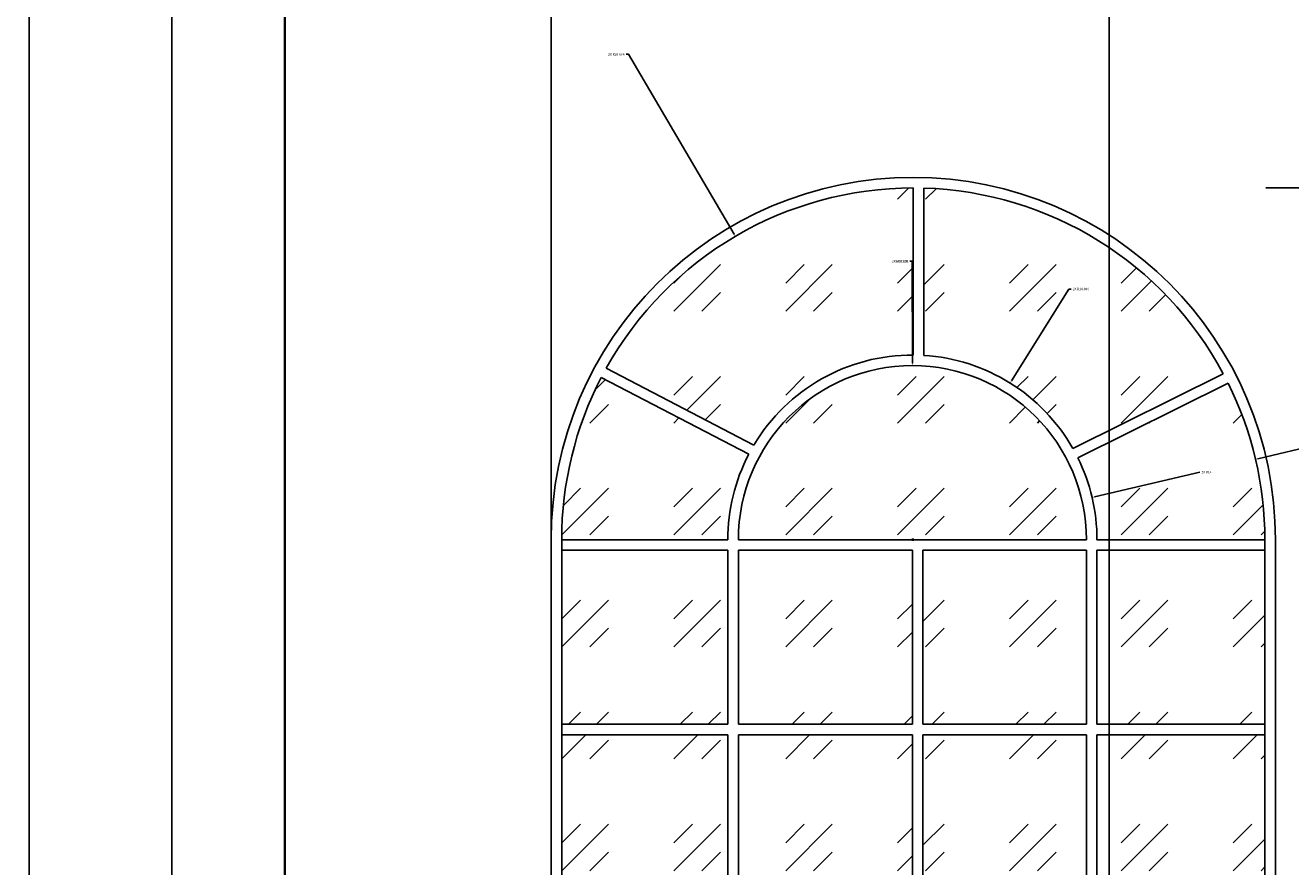
# Model space of a CAD drawing. Units: inches. Extents: x 93 to 565, y 123 to 656.
# Tile 15 of 18: x 418 to 513, y 518 to 582. Entities that reach past the tile are written whole.
import ezdxf

# ---------------------------------------------------------------- set-up
doc = ezdxf.new("R2010")
doc.units = ezdxf.units.IN
doc.header["$MEASUREMENT"] = 0
for name, color, linetype, lineweight in [('A-ANNO-DIMS', 2, 'Continuous', 18), ('A-ELEV', 7, 'Continuous', 35), ('A-GLAZ', 4, 'Continuous', 25)]:
    doc.layers.add(name, color=color, linetype=linetype, lineweight=lineweight)
doc.styles.get("Standard").update_dxf_attribs({"font": 'arial.ttf'})
doc.dimstyles.get("Standard").update_dxf_attribs({"dimtxt": 0.18, "dimasz": 0.18, "dimexe": 0.18, "dimexo": 0.0625, "dimgap": 0.09, "dimtad": 0, "dimtih": 1, "dimtoh": 1, "dimdec": 4, "dimzin": 0, "dimdsep": 46, "dimtxsty": 'Standard', "dimcen": 0.09, "dimadec": 0, "dimazin": 0, "dimtfac": 1, "dimtdec": 4, "dimtofl": 0, "dimtmove": 0, "dimatfit": 3, "dimfxl": 1, "dimtolj": 1, "dimtzin": 0, "dimarcsym": 0})

# ---------------------------------------------------------------- blocks, each defined once
blk = doc.blocks.new('WIN-ARCHED')
for p, q in [((26.666, 83.051), (26.666, 70.384)), ((27.466, 83.039), (27.466, 70.358)), ((3.385, 69.387), (14.576, 63.554)), ((3.006, 68.683), (14.186, 62.855)), ((50.181, 68.96), (38.77, 63.306)), ((50.548, 68.249), (39.145, 62.599)), ((0, 56.384), (12.6, 56.384)), ((0, 56.384), (0.2, 56.384)), ((0, 56.384), (0, 32.384)), ((13.4, 56.384), (39.8, 56.384)), ((40.6, 56.384), (53.333, 56.384)), ((0, 55.584), (12.6, 55.584)), ((12.6, 55.584), (12.6, 42.384)), ((13.4, 55.584), (13.4, 42.384)), ((13.4, 55.584), (26.6, 55.584)), ((26.6, 55.584), (26.6, 42.384)), ((27.4, 55.584), (27.4, 42.384)), ((27.4, 55.584), (39.8, 55.584)), ((39.8, 55.584), (39.8, 42.384)), ((40.6, 55.584), (40.6, 42.384)), ((40.6, 55.584), (53.333, 55.584)), ((0, 42.384), (12.6, 42.384)), ((13.4, 42.384), (26.6, 42.384)), ((27.4, 42.384), (39.8, 42.384)), ((40.6, 42.384), (53.333, 42.384)), ((0, 41.584), (12.6, 41.584)), ((12.6, 41.584), (12.6, 28.384)), ((13.4, 41.584), (13.4, 28.384)), ((13.4, 41.584), (26.6, 41.584)), ((26.6, 41.584), (26.6, 28.384)), ((27.4, 41.584), (27.4, 28.384)), ((27.4, 41.584), (39.8, 41.584)), ((39.8, 41.584), (39.8, 28.384)), ((40.6, 41.584), (40.6, 28.384)), ((40.6, 41.584), (53.333, 41.584)), ((0, 28.384), (12.6, 28.384)), ((13.4, 28.384), (26.6, 28.384)), ((27.4, 28.384), (39.8, 28.384)), ((40.6, 28.384), (53.333, 28.384)), ((0, 27.584), (12.6, 27.584)), ((12.6, 27.584), (12.6, 14.384)), ((13.4, 27.584), (13.4, 14.384)), ((13.4, 27.584), (26.6, 27.584)), ((26.6, 27.584), (26.6, 14.384)), ((27.4, 27.584), (27.4, 14.384)), ((27.4, 27.584), (39.8, 27.584)), ((39.8, 27.584), (39.8, 14.384)), ((40.6, 27.584), (40.6, 14.384)), ((40.6, 27.584), (53.333, 27.584)), ((0, 14.384), (12.6, 14.384)), ((0, 13.584), (12.6, 13.584)), ((12.6, 13.584), (12.6, 0)), ((13.4, 14.384), (26.6, 14.384)), ((13.4, 13.584), (13.4, 0)), ((13.4, 13.584), (26.6, 13.584)), ((26.6, 13.584), (26.6, 0)), ((27.4, 14.384), (39.8, 14.384)), ((27.4, 13.584), (27.4, 0)), ((27.4, 13.584), (39.8, 13.584)), ((39.8, 13.584), (39.8, 0)), ((40.6, 14.384), (53.333, 14.384)), ((40.6, 13.584), (40.6, 0)), ((40.6, 13.584), (53.333, 13.584))]:
    blk.add_line(p, q)
blk.add_lwpolyline([(53.333, 56.384), (53.333, 0), (0, 0), (0, 56.384)])
for centre, radius, start, end in [((26.666, 56.384), 26.666, 90, 150.81666), ((26.666, 56.384), 26.666, 28.13721, 88.28084), ((26.6, 56.384), 14, 89.72913, 149.19423), ((26.6, 56.384), 14, 29.63071, 86.45282), ((26.6, 56.384), 13.2, 0, 180), ((26.666, 56.384), 26.666, 152.53579, 180), ((26.666, 56.384), 26.666, 0, 26.41802), ((26.6, 56.384), 14, 152.47006, 180), ((26.6, 56.384), 14, 0, 26.35489)]:
    blk.add_arc(centre, radius, start, end)
blk = doc.blocks.new('*D20')
at = {"layer": 'A-ANNO-DIMS', "color": 0, "lineweight": -2, "transparency": 16777216}
for p, q in [((511.588, 569.373), (524.163, 569.373)), ((523.983, 569.193), (523.983, 528.031)), ((523.983, 486.502), (523.983, 527.664)), ((511.588, 486.322), (524.163, 486.322))]:
    blk.add_line(p, q, dxfattribs=at)
at = {"layer": 'A-ANNO-DIMS', "color": 0, "transparency": 16777216}
for points in [[(523.953, 569.193), (524.013, 569.193), (523.983, 569.373)], [(523.953, 486.502), (524.013, 486.502), (523.983, 486.322)]]:
    blk.add_solid(points, dxfattribs=at)
at = {"layer": 'Defpoints', "color": 0, "transparency": 16777216}
for p in [(511.526, 569.373), (523.983, 569.373), (511.526, 486.322)]:
    blk.add_point(p, dxfattribs=at)
at = {"layer": 'A-ANNO-DIMS', "color": 0, "transparency": 16777216, "insert": (523.983, 527.847), "char_height": 0.18, "attachment_point": 5}
blk.add_mtext('\\A1;ARCHED WINDOW 83 TYP.', dxfattribs=at)
blk = doc.blocks.new('*D26')
at = {"layer": 'A-ANNO-DIMS', "color": 0, "lineweight": -2, "transparency": 16777216}
for p, q in [((119.079, 519.162), (119.079, 656.135)), ((119.259, 655.955), (328.787, 655.955)), ((538.899, 655.955), (329.372, 655.955)), ((539.079, 630.467), (539.079, 656.135))]:
    blk.add_line(p, q, dxfattribs=at)
at = {"layer": 'A-ANNO-DIMS', "color": 0, "transparency": 16777216}
for points in [[(119.259, 655.985), (119.259, 655.925), (119.079, 655.955)], [(538.899, 655.985), (538.899, 655.925), (539.079, 655.955)]]:
    blk.add_solid(points, dxfattribs=at)
at = {"layer": 'Defpoints', "color": 0, "transparency": 16777216}
for p in [(539.079, 655.955), (539.079, 630.405), (119.079, 519.1)]:
    blk.add_point(p, dxfattribs=at)
at = {"layer": 'A-ANNO-DIMS', "color": 0, "transparency": 16777216, "insert": (329.079, 655.955), "char_height": 0.18, "attachment_point": 5}
blk.add_mtext('\\A1;420', dxfattribs=at)
blk = doc.blocks.new('*D29')
at = {"layer": 'A-ANNO-DIMS', "color": 0, "lineweight": -2, "transparency": 16777216}
for p, q in [((437.189, 594.342), (437.189, 134.002)), ((295.687, 183.67), (295.687, 134.002)), ((295.867, 134.182), (366.052, 134.182)), ((437.009, 134.182), (366.824, 134.182))]:
    blk.add_line(p, q, dxfattribs=at)
at = {"layer": 'A-ANNO-DIMS', "color": 0, "transparency": 16777216}
for points in [[(295.867, 134.212), (295.867, 134.152), (295.687, 134.182)], [(437.009, 134.212), (437.009, 134.152), (437.189, 134.182)]]:
    blk.add_solid(points, dxfattribs=at)
at = {"layer": 'Defpoints', "color": 0, "transparency": 16777216}
for p in [(437.189, 594.405), (295.687, 183.732), (437.189, 134.182)]:
    blk.add_point(p, dxfattribs=at)
at = {"layer": 'A-ANNO-DIMS', "color": 0, "transparency": 16777216, "insert": (366.438, 134.182), "char_height": 0.18, "attachment_point": 5}
blk.add_mtext('\\A1;141.5', dxfattribs=at)
blk = doc.blocks.new('*D30')
at = {"layer": 'A-ANNO-DIMS', "color": 0, "lineweight": -2, "transparency": 16777216}
for p, q in [((437.189, 594.342), (437.189, 134.002)), ((539.079, 159.67), (539.079, 134.002)), ((437.369, 134.182), (487.749, 134.182)), ((538.899, 134.182), (488.519, 134.182))]:
    blk.add_line(p, q, dxfattribs=at)
at = {"layer": 'A-ANNO-DIMS', "color": 0, "transparency": 16777216}
for points in [[(437.369, 134.212), (437.369, 134.152), (437.189, 134.182)], [(538.899, 134.212), (538.899, 134.152), (539.079, 134.182)]]:
    blk.add_solid(points, dxfattribs=at)
at = {"layer": 'Defpoints', "color": 0, "transparency": 16777216}
for p in [(437.189, 594.405), (539.079, 159.732), (539.079, 134.182)]:
    blk.add_point(p, dxfattribs=at)
at = {"layer": 'A-ANNO-DIMS', "color": 0, "transparency": 16777216, "insert": (488.134, 134.182), "char_height": 0.18, "attachment_point": 5}
blk.add_mtext('\\A1;101.9', dxfattribs=at)
blk = doc.blocks.new('*D31')
at = {"layer": 'A-ANNO-DIMS', "color": 0, "lineweight": -2, "transparency": 16777216}
for p, q in [((417.872, 630.405), (564.809, 630.405)), ((564.629, 630.225), (564.629, 395.25)), ((564.629, 159.912), (564.629, 394.887)), ((119.142, 159.732), (564.809, 159.732))]:
    blk.add_line(p, q, dxfattribs=at)
at = {"layer": 'A-ANNO-DIMS', "color": 0, "transparency": 16777216}
for points in [[(564.599, 630.225), (564.659, 630.225), (564.629, 630.405)], [(564.599, 159.912), (564.659, 159.912), (564.629, 159.732)]]:
    blk.add_solid(points, dxfattribs=at)
at = {"layer": 'Defpoints', "color": 0, "transparency": 16777216}
for p in [(417.81, 630.405), (564.629, 630.405), (119.079, 159.732)]:
    blk.add_point(p, dxfattribs=at)
at = {"layer": 'A-ANNO-DIMS', "color": 0, "transparency": 16777216, "insert": (564.629, 395.069), "char_height": 0.18, "attachment_point": 5}
blk.add_mtext('\\A1;470.7', dxfattribs=at)
blk = doc.blocks.new('*D36')
at = {"layer": 'A-ANNO-DIMS', "color": 0, "lineweight": -2, "transparency": 16777216}
for p, q in [((417.747, 594.405), (93.349, 594.405)), ((93.529, 594.225), (93.529, 556.934)), ((93.529, 519.28), (93.529, 556.57)), ((119.017, 519.1), (93.349, 519.1))]:
    blk.add_line(p, q, dxfattribs=at)
at = {"layer": 'A-ANNO-DIMS', "color": 0, "transparency": 16777216}
for points in [[(93.499, 594.225), (93.559, 594.225), (93.529, 594.405)], [(93.499, 519.28), (93.559, 519.28), (93.529, 519.1)]]:
    blk.add_solid(points, dxfattribs=at)
at = {"layer": 'Defpoints', "color": 0, "transparency": 16777216}
for p in [(93.529, 594.405), (417.81, 594.405), (119.079, 519.1)]:
    blk.add_point(p, dxfattribs=at)
at = {"layer": 'A-ANNO-DIMS', "color": 0, "transparency": 16777216, "insert": (93.529, 556.752), "char_height": 0.18, "attachment_point": 5}
blk.add_mtext('\\A1;75.3', dxfattribs=at)
blk = doc.blocks.new('*D69')
at = {"layer": 'A-ANNO-DIMS', "color": 0, "lineweight": -2, "transparency": 16777216}
for p, q in [((355.46, 420.63), (355.46, 656.135)), ((355.64, 655.955), (391.645, 655.955)), ((428.436, 655.955), (392.431, 655.955)), ((428.616, 420.63), (428.616, 656.135))]:
    blk.add_line(p, q, dxfattribs=at)
at = {"layer": 'A-ANNO-DIMS', "color": 0, "transparency": 16777216}
for points in [[(355.64, 655.985), (355.64, 655.925), (355.46, 655.955)], [(428.436, 655.985), (428.436, 655.925), (428.616, 655.955)]]:
    blk.add_solid(points, dxfattribs=at)
at = {"layer": 'Defpoints', "color": 0, "transparency": 16777216}
for p in [(428.616, 655.955), (355.46, 420.567), (428.616, 420.567)]:
    blk.add_point(p, dxfattribs=at)
at = {"layer": 'A-ANNO-DIMS', "color": 0, "transparency": 16777216, "insert": (392.038, 655.955), "char_height": 0.18, "attachment_point": 5}
blk.add_mtext('\\A1;73.16', dxfattribs=at)
blk = doc.blocks.new('*D76')
at = {"layer": 'A-ANNO-DIMS', "color": 0, "lineweight": -2, "transparency": 16777216}
for p, q in [((399.695, 507.892), (399.695, 656.135)), ((399.875, 655.955), (417.978, 655.955)), ((437.009, 655.955), (418.905, 655.955)), ((437.189, 507.795), (437.189, 656.135))]:
    blk.add_line(p, q, dxfattribs=at)
at = {"layer": 'A-ANNO-DIMS', "color": 0, "transparency": 16777216}
for points in [[(399.875, 655.985), (399.875, 655.925), (399.695, 655.955)], [(437.009, 655.985), (437.009, 655.925), (437.189, 655.955)]]:
    blk.add_solid(points, dxfattribs=at)
at = {"layer": 'Defpoints', "color": 0, "transparency": 16777216}
for p in [(437.189, 655.955), (399.695, 507.83), (437.189, 507.732)]:
    blk.add_point(p, dxfattribs=at)
at = {"layer": 'A-ANNO-DIMS', "color": 0, "transparency": 16777216, "insert": (418.442, 655.955), "char_height": 0.18, "attachment_point": 5}
blk.add_mtext('\\A1;37.494', dxfattribs=at)
blk = doc.blocks.new('*D82')
at = {"layer": 'A-ANNO-DIMS', "color": 0, "lineweight": -2, "transparency": 16777216}
for p, q in [((437.189, 447.795), (437.189, 656.135)), ((437.369, 655.955), (446.825, 655.955)), ((457.213, 655.955), (447.757, 655.955)), ((457.393, 378.4), (457.393, 656.135))]:
    blk.add_line(p, q, dxfattribs=at)
at = {"layer": 'A-ANNO-DIMS', "color": 0, "transparency": 16777216}
for points in [[(437.369, 655.985), (437.369, 655.925), (437.189, 655.955)], [(457.213, 655.985), (457.213, 655.925), (457.393, 655.955)]]:
    blk.add_solid(points, dxfattribs=at)
at = {"layer": 'Defpoints', "color": 0, "transparency": 16777216}
for p in [(457.393, 655.955), (437.189, 447.732), (457.393, 378.337)]:
    blk.add_point(p, dxfattribs=at)
at = {"layer": 'A-ANNO-DIMS', "color": 0, "transparency": 16777216, "insert": (447.291, 655.955), "char_height": 0.18, "attachment_point": 5}
blk.add_mtext('\\A1;20.205', dxfattribs=at)
blk = doc.blocks.new('*D90')
at = {"layer": 'A-ANNO-DIMS', "color": 0, "lineweight": -2, "transparency": 16777216}
for p, q in [((417.81, 594.342), (417.81, 134.002)), ((437.189, 594.342), (437.189, 134.002)), ((417.99, 134.182), (427.114, 134.182)), ((437.009, 134.182), (427.885, 134.182))]:
    blk.add_line(p, q, dxfattribs=at)
at = {"layer": 'A-ANNO-DIMS', "color": 0, "transparency": 16777216}
for points in [[(417.99, 134.212), (417.99, 134.152), (417.81, 134.182)], [(437.009, 134.212), (437.009, 134.152), (437.189, 134.182)]]:
    blk.add_solid(points, dxfattribs=at)
at = {"layer": 'Defpoints', "color": 0, "transparency": 16777216}
for p in [(417.81, 594.405), (437.189, 594.405), (437.189, 134.182)]:
    blk.add_point(p, dxfattribs=at)
at = {"layer": 'A-ANNO-DIMS', "color": 0, "transparency": 16777216, "insert": (427.499, 134.182), "char_height": 0.18, "attachment_point": 5}
blk.add_mtext('\\A1;19.38', dxfattribs=at)
blk = doc.blocks.new('*D91')
at = {"layer": 'A-ANNO-DIMS', "color": 0, "lineweight": -2, "transparency": 16777216}
for p, q in [((499.729, 599.755), (499.729, 134.002)), ((437.189, 594.342), (437.189, 134.002)), ((437.369, 134.182), (468.065, 134.182)), ((499.549, 134.182), (468.853, 134.182))]:
    blk.add_line(p, q, dxfattribs=at)
at = {"layer": 'A-ANNO-DIMS', "color": 0, "transparency": 16777216}
for points in [[(437.369, 134.212), (437.369, 134.152), (437.189, 134.182)], [(499.549, 134.212), (499.549, 134.152), (499.729, 134.182)]]:
    blk.add_solid(points, dxfattribs=at)
at = {"layer": 'Defpoints', "color": 0, "transparency": 16777216}
for p in [(499.729, 599.817), (437.189, 594.405), (499.729, 134.182)]:
    blk.add_point(p, dxfattribs=at)
at = {"layer": 'A-ANNO-DIMS', "color": 0, "transparency": 16777216, "insert": (468.459, 134.182), "char_height": 0.18, "attachment_point": 5}
blk.add_mtext('\\A1;62.54', dxfattribs=at)
blk = doc.blocks.new('*D92')
at = {"layer": 'A-ANNO-DIMS', "color": 0, "lineweight": -2, "transparency": 16777216}
for p, q in [((523.142, 603.135), (523.142, 134.002)), ((499.729, 599.755), (499.729, 134.002)), ((499.909, 134.182), (510.971, 134.182)), ((522.962, 134.182), (511.9, 134.182))]:
    blk.add_line(p, q, dxfattribs=at)
at = {"layer": 'A-ANNO-DIMS', "color": 0, "transparency": 16777216}
for points in [[(499.909, 134.212), (499.909, 134.152), (499.729, 134.182)], [(522.962, 134.212), (522.962, 134.152), (523.142, 134.182)]]:
    blk.add_solid(points, dxfattribs=at)
at = {"layer": 'Defpoints', "color": 0, "transparency": 16777216}
for p in [(523.142, 603.198), (499.729, 599.817), (523.142, 134.182)]:
    blk.add_point(p, dxfattribs=at)
at = {"layer": 'A-ANNO-DIMS', "color": 0, "transparency": 16777216, "insert": (511.435, 134.182), "char_height": 0.18, "attachment_point": 5}
blk.add_mtext('\\A1;23.412', dxfattribs=at)
blk = doc.blocks.new('*D102')
at = {"layer": 'A-ANNO-DIMS', "color": 0, "lineweight": -2, "transparency": 16777216}
for p, q in [((526.396, 552.456), (510.995, 548.841)), ((484.769, 542.706), (484.949, 542.706)), ((484.859, 542.616), (484.859, 542.796))]:
    blk.add_line(p, q, dxfattribs=at)
at = {"layer": 'A-ANNO-DIMS', "color": 0, "transparency": 16777216}
blk.add_solid([(510.988, 548.87), (511.002, 548.812), (510.82, 548.8)], dxfattribs=at)
at = {"layer": 'Defpoints', "color": 0, "transparency": 16777216}
for p in [(510.82, 548.8), (484.859, 542.706)]:
    blk.add_point(p, dxfattribs=at)
at = {"layer": 'A-ANNO-DIMS', "color": 0, "transparency": 16777216, "insert": (527.141, 552.456), "char_height": 0.18, "attachment_point": 5}
blk.add_mtext('\\A1;2X R26.666', dxfattribs=at)
blk = doc.blocks.new('*D103')
at = {"layer": 'A-ANNO-DIMS', "color": 0, "lineweight": -2, "transparency": 16777216}
for p, q in [((506.601, 547.825), (498.598, 545.947)), ((484.703, 542.706), (484.883, 542.706)), ((484.793, 542.616), (484.793, 542.796))]:
    blk.add_line(p, q, dxfattribs=at)
at = {"layer": 'A-ANNO-DIMS', "color": 0, "transparency": 16777216}
blk.add_solid([(498.591, 545.976), (498.605, 545.917), (498.423, 545.905)], dxfattribs=at)
at = {"layer": 'Defpoints', "color": 0, "transparency": 16777216}
for p in [(498.423, 545.905), (484.793, 542.706)]:
    blk.add_point(p, dxfattribs=at)
at = {"layer": 'A-ANNO-DIMS', "color": 0, "transparency": 16777216, "insert": (507.1, 547.825), "char_height": 0.18, "attachment_point": 5}
blk.add_mtext('\\A1;2X R14', dxfattribs=at)
blk = doc.blocks.new('*D104')
at = {"layer": 'A-ANNO-DIMS', "color": 0, "lineweight": -2, "transparency": 16777216}
for p, q in [((484.608, 563.826), (484.788, 563.826)), ((484.788, 563.826), (484.79, 556.086)), ((484.703, 542.706), (484.883, 542.706)), ((484.793, 542.616), (484.793, 542.796))]:
    blk.add_line(p, q, dxfattribs=at)
at = {"layer": 'A-ANNO-DIMS', "color": 0, "transparency": 16777216}
blk.add_solid([(484.82, 556.086), (484.76, 556.086), (484.79, 555.906)], dxfattribs=at)
at = {"layer": 'Defpoints', "color": 0, "transparency": 16777216}
for p in [(484.79, 555.906), (484.793, 542.706)]:
    blk.add_point(p, dxfattribs=at)
at = {"layer": 'A-ANNO-DIMS', "color": 0, "transparency": 16777216, "insert": (484.004, 563.826), "char_height": 0.18, "attachment_point": 5}
blk.add_mtext('\\A1;2X R13.2', dxfattribs=at)
blk = doc.blocks.new('*D105')
at = {"layer": 'A-ANNO-DIMS', "color": 0, "lineweight": -2, "transparency": 16777216}
for p, q in [((119.079, 519.162), (119.079, 656.135)), ((119.259, 655.955), (328.542, 655.955)), ((538.899, 655.955), (329.616, 655.955)), ((539.079, 630.467), (539.079, 656.135))]:
    blk.add_line(p, q, dxfattribs=at)
at = {"layer": 'A-ANNO-DIMS', "color": 0, "transparency": 16777216}
for points in [[(119.259, 655.985), (119.259, 655.925), (119.079, 655.955)], [(538.899, 655.985), (538.899, 655.925), (539.079, 655.955)]]:
    blk.add_solid(points, dxfattribs=at)
at = {"layer": 'Defpoints', "color": 0, "transparency": 16777216}
for p in [(539.079, 655.955), (539.079, 630.405), (119.079, 519.1)]:
    blk.add_point(p, dxfattribs=at)
at = {"layer": 'A-ANNO-DIMS', "color": 0, "transparency": 16777216, "insert": (329.079, 655.955), "char_height": 0.18, "attachment_point": 5}
blk.add_mtext('\\A1;420.000', dxfattribs=at)
blk = doc.blocks.new('*D108')
at = {"layer": 'A-ANNO-DIMS', "color": 0, "lineweight": -2, "transparency": 16777216}
for p, q in [((437.189, 594.342), (437.189, 134.002)), ((295.687, 183.67), (295.687, 134.002)), ((295.867, 134.182), (365.93, 134.182)), ((437.009, 134.182), (366.946, 134.182))]:
    blk.add_line(p, q, dxfattribs=at)
at = {"layer": 'A-ANNO-DIMS', "color": 0, "transparency": 16777216}
for points in [[(295.867, 134.212), (295.867, 134.152), (295.687, 134.182)], [(437.009, 134.212), (437.009, 134.152), (437.189, 134.182)]]:
    blk.add_solid(points, dxfattribs=at)
at = {"layer": 'Defpoints', "color": 0, "transparency": 16777216}
for p in [(437.189, 594.405), (295.687, 183.732), (437.189, 134.182)]:
    blk.add_point(p, dxfattribs=at)
at = {"layer": 'A-ANNO-DIMS', "color": 0, "transparency": 16777216, "insert": (366.438, 134.182), "char_height": 0.18, "attachment_point": 5}
blk.add_mtext('\\A1;141.501', dxfattribs=at)
blk = doc.blocks.new('*D109')
at = {"layer": 'A-ANNO-DIMS', "color": 0, "lineweight": -2, "transparency": 16777216}
for p, q in [((437.189, 594.342), (437.189, 134.002)), ((539.079, 159.67), (539.079, 134.002)), ((437.369, 134.182), (487.626, 134.182)), ((538.899, 134.182), (488.642, 134.182))]:
    blk.add_line(p, q, dxfattribs=at)
at = {"layer": 'A-ANNO-DIMS', "color": 0, "transparency": 16777216}
for points in [[(437.369, 134.212), (437.369, 134.152), (437.189, 134.182)], [(538.899, 134.212), (538.899, 134.152), (539.079, 134.182)]]:
    blk.add_solid(points, dxfattribs=at)
at = {"layer": 'Defpoints', "color": 0, "transparency": 16777216}
for p in [(437.189, 594.405), (539.079, 159.732), (539.079, 134.182)]:
    blk.add_point(p, dxfattribs=at)
at = {"layer": 'A-ANNO-DIMS', "color": 0, "transparency": 16777216, "insert": (488.134, 134.182), "char_height": 0.18, "attachment_point": 5}
blk.add_mtext('\\A1;101.891', dxfattribs=at)
blk = doc.blocks.new('*D110')
at = {"layer": 'A-ANNO-DIMS', "color": 0, "lineweight": -2, "transparency": 16777216}
for p, q in [((417.872, 630.405), (564.809, 630.405)), ((564.629, 630.225), (564.629, 395.25)), ((564.629, 159.912), (564.629, 394.887)), ((119.142, 159.732), (564.809, 159.732))]:
    blk.add_line(p, q, dxfattribs=at)
at = {"layer": 'A-ANNO-DIMS', "color": 0, "transparency": 16777216}
for points in [[(564.599, 630.225), (564.659, 630.225), (564.629, 630.405)], [(564.599, 159.912), (564.659, 159.912), (564.629, 159.732)]]:
    blk.add_solid(points, dxfattribs=at)
at = {"layer": 'Defpoints', "color": 0, "transparency": 16777216}
for p in [(417.81, 630.405), (564.629, 630.405), (119.079, 159.732)]:
    blk.add_point(p, dxfattribs=at)
at = {"layer": 'A-ANNO-DIMS', "color": 0, "transparency": 16777216, "insert": (564.629, 395.069), "char_height": 0.18, "attachment_point": 5}
blk.add_mtext('\\A1;470.673', dxfattribs=at)
blk = doc.blocks.new('*D115')
at = {"layer": 'A-ANNO-DIMS', "color": 0, "lineweight": -2, "transparency": 16777216}
for p, q in [((417.747, 594.405), (93.349, 594.405)), ((93.529, 594.225), (93.529, 556.934)), ((93.529, 519.28), (93.529, 556.57)), ((119.017, 519.1), (93.349, 519.1))]:
    blk.add_line(p, q, dxfattribs=at)
at = {"layer": 'A-ANNO-DIMS', "color": 0, "transparency": 16777216}
for points in [[(93.499, 594.225), (93.559, 594.225), (93.529, 594.405)], [(93.499, 519.28), (93.559, 519.28), (93.529, 519.1)]]:
    blk.add_solid(points, dxfattribs=at)
at = {"layer": 'Defpoints', "color": 0, "transparency": 16777216}
for p in [(93.529, 594.405), (417.81, 594.405), (119.079, 519.1)]:
    blk.add_point(p, dxfattribs=at)
at = {"layer": 'A-ANNO-DIMS', "color": 0, "transparency": 16777216, "insert": (93.529, 556.752), "char_height": 0.18, "attachment_point": 5}
blk.add_mtext('\\A1;75.305', dxfattribs=at)
blk = doc.blocks.new('*D148')
at = {"layer": 'A-ANNO-DIMS', "color": 0, "lineweight": -2, "transparency": 16777216}
for p, q in [((355.46, 420.63), (355.46, 656.135)), ((355.64, 655.955), (391.575, 655.955)), ((428.436, 655.955), (392.501, 655.955)), ((428.616, 420.63), (428.616, 656.135))]:
    blk.add_line(p, q, dxfattribs=at)
at = {"layer": 'A-ANNO-DIMS', "color": 0, "transparency": 16777216}
for points in [[(355.64, 655.985), (355.64, 655.925), (355.46, 655.955)], [(428.436, 655.985), (428.436, 655.925), (428.616, 655.955)]]:
    blk.add_solid(points, dxfattribs=at)
at = {"layer": 'Defpoints', "color": 0, "transparency": 16777216}
for p in [(428.616, 655.955), (355.46, 420.567), (428.616, 420.567)]:
    blk.add_point(p, dxfattribs=at)
at = {"layer": 'A-ANNO-DIMS', "color": 0, "transparency": 16777216, "insert": (392.038, 655.955), "char_height": 0.18, "attachment_point": 5}
blk.add_mtext('\\A1;73.156', dxfattribs=at)
blk = doc.blocks.new('*D155')
at = {"layer": 'A-ANNO-DIMS', "color": 0, "lineweight": -2, "transparency": 16777216}
for p, q in [((399.695, 507.892), (399.695, 656.135)), ((399.875, 655.955), (417.978, 655.955)), ((437.009, 655.955), (418.905, 655.955)), ((437.189, 507.795), (437.189, 656.135))]:
    blk.add_line(p, q, dxfattribs=at)
at = {"layer": 'A-ANNO-DIMS', "color": 0, "transparency": 16777216}
for points in [[(399.875, 655.985), (399.875, 655.925), (399.695, 655.955)], [(437.009, 655.985), (437.009, 655.925), (437.189, 655.955)]]:
    blk.add_solid(points, dxfattribs=at)
at = {"layer": 'Defpoints', "color": 0, "transparency": 16777216}
for p in [(437.189, 655.955), (399.695, 507.83), (437.189, 507.732)]:
    blk.add_point(p, dxfattribs=at)
at = {"layer": 'A-ANNO-DIMS', "color": 0, "transparency": 16777216, "insert": (418.442, 655.955), "char_height": 0.18, "attachment_point": 5}
blk.add_mtext('\\A1;37.494', dxfattribs=at)
blk = doc.blocks.new('*D161')
at = {"layer": 'A-ANNO-DIMS', "color": 0, "lineweight": -2, "transparency": 16777216}
for p, q in [((437.189, 447.795), (437.189, 656.135)), ((437.369, 655.955), (446.825, 655.955)), ((457.213, 655.955), (447.757, 655.955)), ((457.393, 378.4), (457.393, 656.135))]:
    blk.add_line(p, q, dxfattribs=at)
at = {"layer": 'A-ANNO-DIMS', "color": 0, "transparency": 16777216}
for points in [[(437.369, 655.985), (437.369, 655.925), (437.189, 655.955)], [(457.213, 655.985), (457.213, 655.925), (457.393, 655.955)]]:
    blk.add_solid(points, dxfattribs=at)
at = {"layer": 'Defpoints', "color": 0, "transparency": 16777216}
for p in [(457.393, 655.955), (437.189, 447.732), (457.393, 378.337)]:
    blk.add_point(p, dxfattribs=at)
at = {"layer": 'A-ANNO-DIMS', "color": 0, "transparency": 16777216, "insert": (447.291, 655.955), "char_height": 0.18, "attachment_point": 5}
blk.add_mtext('\\A1;20.205', dxfattribs=at)
blk = doc.blocks.new('*D169')
at = {"layer": 'A-ANNO-DIMS', "color": 0, "lineweight": -2, "transparency": 16777216}
for p, q in [((417.81, 594.342), (417.81, 134.002)), ((437.189, 594.342), (437.189, 134.002)), ((417.99, 134.182), (427.044, 134.182)), ((437.009, 134.182), (427.954, 134.182))]:
    blk.add_line(p, q, dxfattribs=at)
at = {"layer": 'A-ANNO-DIMS', "color": 0, "transparency": 16777216}
for points in [[(417.99, 134.212), (417.99, 134.152), (417.81, 134.182)], [(437.009, 134.212), (437.009, 134.152), (437.189, 134.182)]]:
    blk.add_solid(points, dxfattribs=at)
at = {"layer": 'Defpoints', "color": 0, "transparency": 16777216}
for p in [(417.81, 594.405), (437.189, 594.405), (437.189, 134.182)]:
    blk.add_point(p, dxfattribs=at)
at = {"layer": 'A-ANNO-DIMS', "color": 0, "transparency": 16777216, "insert": (427.499, 134.182), "char_height": 0.18, "attachment_point": 5}
blk.add_mtext('\\A1;19.379', dxfattribs=at)
blk = doc.blocks.new('*D170')
at = {"layer": 'A-ANNO-DIMS', "color": 0, "lineweight": -2, "transparency": 16777216}
for p, q in [((499.729, 599.755), (499.729, 134.002)), ((437.189, 594.342), (437.189, 134.002)), ((437.369, 134.182), (468.012, 134.182)), ((499.549, 134.182), (468.906, 134.182))]:
    blk.add_line(p, q, dxfattribs=at)
at = {"layer": 'A-ANNO-DIMS', "color": 0, "transparency": 16777216}
for points in [[(437.369, 134.212), (437.369, 134.152), (437.189, 134.182)], [(499.549, 134.212), (499.549, 134.152), (499.729, 134.182)]]:
    blk.add_solid(points, dxfattribs=at)
at = {"layer": 'Defpoints', "color": 0, "transparency": 16777216}
for p in [(499.729, 599.817), (437.189, 594.405), (499.729, 134.182)]:
    blk.add_point(p, dxfattribs=at)
at = {"layer": 'A-ANNO-DIMS', "color": 0, "transparency": 16777216, "insert": (468.459, 134.182), "char_height": 0.18, "attachment_point": 5}
blk.add_mtext('\\A1;62.541', dxfattribs=at)
blk = doc.blocks.new('*D171')
at = {"layer": 'A-ANNO-DIMS', "color": 0, "lineweight": -2, "transparency": 16777216}
for p, q in [((523.142, 603.135), (523.142, 134.002)), ((499.729, 599.755), (499.729, 134.002)), ((499.909, 134.182), (510.971, 134.182)), ((522.962, 134.182), (511.9, 134.182))]:
    blk.add_line(p, q, dxfattribs=at)
at = {"layer": 'A-ANNO-DIMS', "color": 0, "transparency": 16777216}
for points in [[(499.909, 134.212), (499.909, 134.152), (499.729, 134.182)], [(522.962, 134.212), (522.962, 134.152), (523.142, 134.182)]]:
    blk.add_solid(points, dxfattribs=at)
at = {"layer": 'Defpoints', "color": 0, "transparency": 16777216}
for p in [(523.142, 603.198), (499.729, 599.817), (523.142, 134.182)]:
    blk.add_point(p, dxfattribs=at)
at = {"layer": 'A-ANNO-DIMS', "color": 0, "transparency": 16777216, "insert": (511.435, 134.182), "char_height": 0.18, "attachment_point": 5}
blk.add_mtext('\\A1;23.412', dxfattribs=at)
blk = doc.blocks.new('*D200')
at = {"layer": 'A-ANNO-DIMS', "color": 0, "lineweight": -2, "transparency": 16777216}
for p, q in [((463.083, 579.503), (463.263, 579.503)), ((463.263, 579.503), (471.271, 565.859)), ((484.769, 542.706), (484.949, 542.706)), ((484.859, 542.616), (484.859, 542.796))]:
    blk.add_line(p, q, dxfattribs=at)
at = {"layer": 'A-ANNO-DIMS', "color": 0, "transparency": 16777216}
blk.add_solid([(471.297, 565.875), (471.245, 565.844), (471.362, 565.704)], dxfattribs=at)
at = {"layer": 'Defpoints', "color": 0, "transparency": 16777216}
for p in [(471.362, 565.704), (484.859, 542.706)]:
    blk.add_point(p, dxfattribs=at)
at = {"layer": 'A-ANNO-DIMS', "color": 0, "transparency": 16777216, "insert": (462.339, 579.503), "char_height": 0.18, "attachment_point": 5}
blk.add_mtext('\\A1;2X R26.666', dxfattribs=at)
blk = doc.blocks.new('*D201')
at = {"layer": 'A-ANNO-DIMS', "color": 0, "lineweight": -2, "transparency": 16777216}
for p, q in [((496.651, 561.711), (492.299, 554.737)), ((496.831, 561.711), (496.651, 561.711)), ((484.703, 542.706), (484.883, 542.706)), ((484.793, 542.616), (484.793, 542.796))]:
    blk.add_line(p, q, dxfattribs=at)
at = {"layer": 'A-ANNO-DIMS', "color": 0, "transparency": 16777216}
blk.add_solid([(492.274, 554.753), (492.325, 554.721), (492.204, 554.584)], dxfattribs=at)
at = {"layer": 'Defpoints', "color": 0, "transparency": 16777216}
for p in [(492.204, 554.584), (484.793, 542.706)]:
    blk.add_point(p, dxfattribs=at)
at = {"layer": 'A-ANNO-DIMS', "color": 0, "transparency": 16777216, "insert": (497.575, 561.711), "char_height": 0.18, "attachment_point": 5}
blk.add_mtext('\\A1;2X R14.000', dxfattribs=at)
blk = doc.blocks.new('*D202')
at = {"layer": 'A-ANNO-DIMS', "color": 0, "lineweight": -2, "transparency": 16777216}
for p, q in [((484.608, 563.826), (484.788, 563.826)), ((484.788, 563.826), (484.79, 556.086)), ((484.703, 542.706), (484.883, 542.706)), ((484.793, 542.616), (484.793, 542.796))]:
    blk.add_line(p, q, dxfattribs=at)
at = {"layer": 'A-ANNO-DIMS', "color": 0, "transparency": 16777216}
blk.add_solid([(484.82, 556.086), (484.76, 556.086), (484.79, 555.906)], dxfattribs=at)
at = {"layer": 'Defpoints', "color": 0, "transparency": 16777216}
for p in [(484.79, 555.906), (484.793, 542.706)]:
    blk.add_point(p, dxfattribs=at)
at = {"layer": 'A-ANNO-DIMS', "color": 0, "transparency": 16777216, "insert": (483.864, 563.826), "char_height": 0.18, "attachment_point": 5}
blk.add_mtext('\\A1;2X R13.200', dxfattribs=at)

msp = doc.modelspace()

# ---------------------------------------------------------------- hatches: boundary and pattern name
at = {"layer": 'A-GLAZ'}
h = msp.add_hatch(dxfattribs=at)
h.set_pattern_fill('GOST_GLASS', color=256)
h.set_pattern_definition([(45, (0, 0), (8.48528, 0), [5, -7]), (45, (2.1213, 0), (8.48528, 0), [2, -10]), (45, (0, 2.1213), (8.48528, 0), [2, -10])])
h.paths.add_polyline_path([(472.3785, 549.1774), (461.1986, 555.0047, 0.1204122), (458.1933, 542.7064), (458.3933, 542.7064), (470.7933, 542.7064, -0.1207031)])
h.paths.add_polyline_path([(470.7933, 541.9064), (458.1933, 541.9064), (458.1933, 528.7064), (470.7933, 528.7064)])
h.paths.add_polyline_path([(470.7933, 527.9064), (458.1933, 527.9064), (458.1933, 518.7064), (458.1933, 514.7064), (470.7933, 514.7064)])
h.paths.add_polyline_path([(470.7933, 513.9064), (458.1933, 513.9064), (458.1933, 500.7064), (470.7933, 500.7064)])
h.paths.add_polyline_path([(470.7933, 499.9064), (458.1933, 499.9064), (458.1933, 486.3222), (470.7933, 486.3222)])
h.paths.add_polyline_path([(484.7933, 499.9064), (471.5933, 499.9064), (471.5933, 486.3222), (484.7933, 486.3222)])
h.paths.add_polyline_path([(484.7933, 513.9064), (471.5933, 513.9064), (471.5933, 500.7064), (484.7933, 500.7064)])
h.paths.add_polyline_path([(484.7933, 527.9064), (471.5933, 527.9064), (471.5933, 514.7064), (484.7933, 514.7064)])
h.paths.add_polyline_path([(484.7933, 541.9064), (471.5933, 541.9064), (471.5933, 528.7064), (484.7933, 528.7064)])
h.paths.add_polyline_path([(497.9933, 541.9064), (485.5933, 541.9064), (485.5933, 528.7064), (497.9933, 528.7064)])
h.paths.add_polyline_path([(497.9933, 527.9064), (485.5933, 527.9064), (485.5933, 514.7064), (497.9933, 514.7064)])
h.paths.add_polyline_path([(497.9933, 513.9064), (485.5933, 513.9064), (485.5933, 500.7064), (497.9933, 500.7064)])
h.paths.add_polyline_path([(497.9933, 499.9064), (485.5933, 499.9064), (485.5933, 486.3222), (497.9933, 486.3222)])
h.paths.add_polyline_path([(511.5257, 499.9064), (498.7933, 499.9064), (498.7933, 486.3222), (511.5257, 486.3222)])
h.paths.add_polyline_path([(511.5257, 513.9064), (498.7933, 513.9064), (498.7933, 500.7064), (511.5257, 500.7064)])
h.paths.add_polyline_path([(511.5257, 527.9064), (498.7933, 527.9064), (498.7933, 514.7064), (511.5257, 514.7064)])
h.paths.add_polyline_path([(511.5257, 541.9064), (498.7933, 541.9064), (498.7933, 528.7064), (511.5257, 528.7064)])
h.paths.add_polyline_path([(471.5933, 542.7064), (497.9933, 542.7064, 1)])
h.paths.add_polyline_path([(508.741, 554.5706), (497.3382, 548.9214, -0.1155045), (498.7933, 542.7064), (511.5257, 542.7064, 0.1157836)])
h.paths.add_polyline_path([(485.6595, 569.3606), (485.6595, 556.6796, -0.2531415), (496.9625, 549.6281), (508.3743, 555.2818, 0.268621)])
h.paths.add_polyline_path([(484.8595, 569.3726, 0.271772), (461.5782, 555.709), (472.7686, 549.8762, -0.2654493), (484.8595, 556.7062)])

# ---------------------------------------------------------------- linework, layer by layer
at = {"layer": 'A-ELEV'}
msp.add_line((437.1885, 594.4048), (437.1885, 507.7323), dxfattribs=at)
at = {"layer": 'A-GLAZ'}
for p, q in [((485.6595, 570.1726), (485.6595, 570.1609)), ((460.859, 556.0839), (460.8685, 556.0789)), ((509.1027, 555.6426), (509.0915, 555.6371)), ((457.3933, 542.7064), (457.3933, 527.1064))]:
    msp.add_line(p, q, dxfattribs=at)
msp.add_lwpolyline([(512.3257, 542.7064), (512.3257, 485.5222), (457.3933, 485.5222), (457.3933, 542.7064)], dxfattribs=at)
msp.add_arc((484.8595, 542.7064), 27.4662, 0, 180, dxfattribs=at)

# ---------------------------------------------------------------- block references
msp.add_blockref('WIN-ARCHED', (458.193, 486.322), dxfattribs=at)

# ---------------------------------------------------------------- dimensions: what is measured, and where the dimension line sits
at = {"layer": 'A-ANNO-DIMS'}
for base, p1, p2, override, picture, middle in [((539.0794, 655.9548), (119.0794, 519.0999), (539.0794, 630.4048), {"dimdec": 0, "dimlfac": 1, "dimrnd": 0, "dimzin": 0, "dimdsep": 46, "dimlunit": 2}, '*D26', (329.0794, 655.9548)), ((539.0794, 655.9548), (119.0794, 519.0999), (539.0794, 630.4048), {"dimdec": 3, "dimlfac": 1, "dimrnd": 0, "dimzin": 0, "dimdsep": 46, "dimlunit": 2}, '*D105', (329.0794, 655.9548)), ((428.6158, 655.9548), (355.4603, 420.5674), (428.6158, 420.5674), {"dimdec": 2, "dimlfac": 1, "dimrnd": 0, "dimzin": 0, "dimdsep": 46, "dimlunit": 2}, '*D69', (392.038, 655.9548)), ((428.615792, 655.954775), (355.460288, 420.567351), (428.615792, 420.567351), {"dimdec": 3, "dimlfac": 1, "dimrnd": 0, "dimzin": 0, "dimdsep": 46, "dimlunit": 2}, '*D148', (392.03804, 655.954775)), ((437.1885, 655.9548), (399.6946, 507.8299), (437.1885, 507.7323), {"dimdec": 3, "dimlfac": 1, "dimrnd": 0, "dimzin": 0, "dimdsep": 46, "dimlunit": 2}, '*D76', (418.4415, 655.9548)), ((437.1885, 655.9548), (399.6946, 507.8299), (437.1885, 507.7323), {"dimdec": 3, "dimlfac": 1, "dimrnd": 0, "dimzin": 0, "dimdsep": 46, "dimlunit": 2}, '*D155', (418.4415, 655.9548)), ((457.3933, 655.9548), (437.1885, 447.7323), (457.3933, 378.3372), {"dimdec": 3, "dimlfac": 1, "dimrnd": 0, "dimzin": 0, "dimdsep": 46, "dimlunit": 2}, '*D82', (447.2909, 655.9548)), ((457.3933, 655.9548), (437.1885, 447.7323), (457.3933, 378.3372), {"dimdec": 3, "dimlfac": 1, "dimrnd": 0, "dimzin": 0, "dimdsep": 46, "dimlunit": 2}, '*D161', (447.2909, 655.9548)), ((523.1415, 134.1823), (499.7291, 599.8171), (523.1415, 603.1979), {"dimdec": 3, "dimlfac": 1, "dimrnd": 0, "dimzin": 0, "dimdsep": 46, "dimlunit": 2}, '*D92', (511.4353, 134.1823)), ((523.1415, 134.1823), (499.7291, 599.8171), (523.1415, 603.1979), {"dimdec": 3, "dimlfac": 1, "dimrnd": 0, "dimzin": 0, "dimdsep": 46, "dimlunit": 2}, '*D171', (511.4353, 134.1823)), ((499.7291, 134.1823), (437.1885, 594.4048), (499.7291, 599.8171), {"dimdec": 2, "dimlfac": 1, "dimrnd": 0, "dimzin": 0, "dimdsep": 46, "dimlunit": 2}, '*D91', (468.4588, 134.1823)), ((499.7291, 134.1823), (437.1885, 594.4048), (499.7291, 599.8171), {"dimdec": 3, "dimlfac": 1, "dimrnd": 0, "dimzin": 0, "dimdsep": 46, "dimlunit": 2}, '*D170', (468.4588, 134.1823)), ((437.1885, 134.1823), (295.6874, 183.7323), (437.1885, 594.4048), {"dimdec": 1, "dimlfac": 1, "dimrnd": 0, "dimzin": 0, "dimdsep": 46, "dimlunit": 2}, '*D29', (366.438, 134.1823)), ((437.1885, 134.1823), (295.6874, 183.7323), (437.1885, 594.4048), {"dimdec": 3, "dimlfac": 1, "dimrnd": 0, "dimzin": 0, "dimdsep": 46, "dimlunit": 2}, '*D108', (366.438, 134.1823)), ((437.1885, 134.1823), (417.8097, 594.4048), (437.1885, 594.4048), {"dimdec": 2, "dimlfac": 1, "dimrnd": 0, "dimzin": 0, "dimdsep": 46, "dimlunit": 2}, '*D90', (427.4991, 134.1823)), ((437.1885, 134.1823), (417.8097, 594.4048), (437.1885, 594.4048), {"dimdec": 3, "dimlfac": 1, "dimrnd": 0, "dimzin": 0, "dimdsep": 46, "dimlunit": 2}, '*D169', (427.4991, 134.1823)), ((539.0794, 134.1823), (437.1885, 594.4048), (539.0794, 159.7323), {"dimdec": 1, "dimlfac": 1, "dimrnd": 0, "dimzin": 0, "dimdsep": 46, "dimlunit": 2}, '*D30', (488.1339, 134.1823)), ((539.0794, 134.1823), (437.1885, 594.4048), (539.0794, 159.7323), {"dimdec": 3, "dimlfac": 1, "dimrnd": 0, "dimzin": 0, "dimdsep": 46, "dimlunit": 2}, '*D109', (488.1339, 134.1823))]:
    dim = msp.add_linear_dim(base=base, p1=p1, p2=p2, dimstyle='Standard', override=override, dxfattribs=at)
    dim.commit()
    dim.dimension.update_dxf_attribs({"geometry": picture, "text_midpoint": middle})
for base, p1, p2, override, picture, middle in [((564.6294, 630.4048), (119.0794, 159.7323), (417.8097, 630.4048), {"dimdec": 1, "dimlfac": 1, "dimrnd": 0, "dimzin": 0, "dimdsep": 46, "dimlunit": 2}, '*D31', (564.6294, 395.0685)), ((564.62936, 630.40478), (119.07936, 159.73225), (417.80971, 630.40477), {"dimdec": 3, "dimlfac": 1, "dimrnd": 0, "dimzin": 0, "dimdsep": 46, "dimlunit": 2}, '*D110', (564.62936, 395.06851)), ((93.5294, 594.4048), (119.0794, 519.0999), (417.8097, 594.4048), {"dimdec": 3, "dimlfac": 1, "dimrnd": 0, "dimzin": 0, "dimdsep": 46, "dimlunit": 2}, '*D115', (93.5294, 556.7523)), ((93.5294, 594.4048), (119.0794, 519.0999), (417.8097, 594.4048), {"dimdec": 1, "dimlfac": 1, "dimrnd": 0, "dimzin": 0, "dimdsep": 46, "dimlunit": 2}, '*D36', (93.5294, 556.7523))]:
    dim = msp.add_linear_dim(base=base, p1=p1, p2=p2, angle=90, dimstyle='Standard', override=override, dxfattribs=at)
    dim.commit()
    dim.dimension.update_dxf_attribs({"geometry": picture, "text_midpoint": middle})
for center, mpoint, override, picture, middle in [((484.8595, 542.7064), (471.3619, 565.7042), {"dimdec": 3, "dimlfac": 1, "dimrnd": 0, "dimzin": 0, "dimdsep": 46, "dimlunit": 2}, '*D200', (462.3387, 579.5029)), ((484.7933, 542.7064), (484.79, 555.9064), {"dimdec": 3, "dimlfac": 1, "dimrnd": 0, "dimzin": 0, "dimdsep": 46, "dimlunit": 2}, '*D202', (483.8636, 563.8264)), ((484.7933, 542.7064), (484.79, 555.9064), {"dimdec": 1, "dimlfac": 1, "dimrnd": 0, "dimzin": 0, "dimdsep": 46, "dimlunit": 2}, '*D104', (484.0041, 563.8264)), ((484.7933, 542.7064), (492.2041, 554.5841), {"dimdec": 3, "dimlfac": 1, "dimrnd": 0, "dimzin": 0, "dimdsep": 46, "dimlunit": 2}, '*D201', (497.5749, 561.7108)), ((484.8595, 542.7064), (510.8201, 548.8), {"dimdec": 3, "dimlfac": 1, "dimrnd": 0, "dimzin": 0, "dimdsep": 46, "dimlunit": 2}, '*D102', (526.3965, 552.4562)), ((484.7933, 542.7064), (498.4229, 545.9054), {"dimdec": 0, "dimlfac": 1, "dimrnd": 0, "dimzin": 0, "dimdsep": 46, "dimlunit": 2}, '*D103', (506.6007, 547.8248))]:
    dim = msp.add_radius_dim(center=center, mpoint=mpoint, text='2X <>', dimstyle='Standard', override=override, dxfattribs=at)
    dim.commit()
    dim.dimension.update_dxf_attribs({"geometry": picture, "text_midpoint": middle, "dimtype": 164})
dim = msp.add_linear_dim(base=(523.9832, 569.3726), p1=(511.5257, 486.3222), p2=(511.5257, 569.3726), angle=90, text='ARCHED WINDOW <> TYP.', dimstyle='Standard', override={"dimdec": 0, "dimrnd": 0, "dimzin": 0, "dimlunit": 2}, dxfattribs=at)
dim.commit()
dim.dimension.update_dxf_attribs({"geometry": '*D20', "text_midpoint": (523.9832, 527.8474)})

doc.saveas('drawing.dxf')
